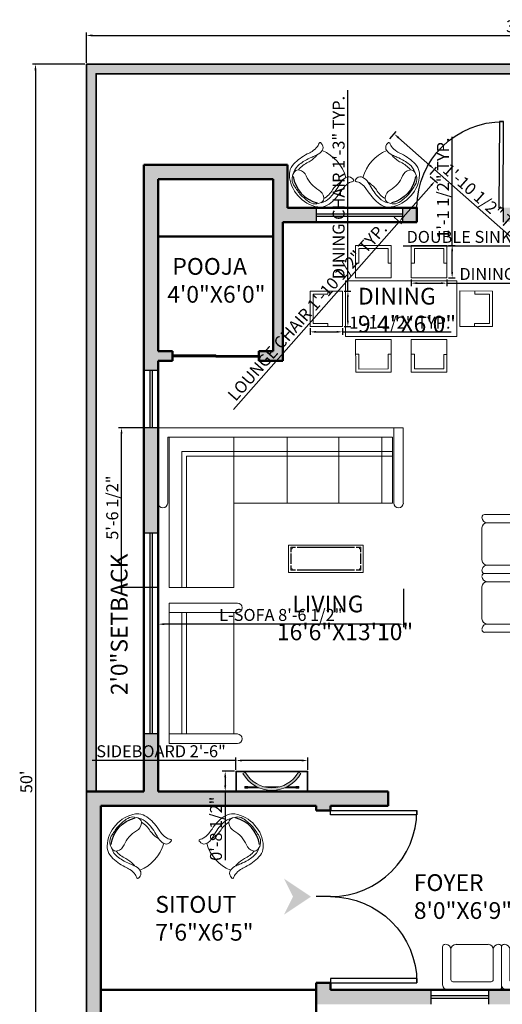
# Model space of a CAD drawing. Units: inches. Extents: x 2638 to 4577, y 1946 to 2619.
# Tile 2 of 8: x 2638 to 2839, y 2207 to 2619. Entities that reach past the tile are written whole.
import ezdxf

# ---------------------------------------------------------------- set-up
doc = ezdxf.new("R2010")
doc.units = ezdxf.units.IN
for name, color, linetype, lineweight in [('A-ANNO-DIMS', 2, 'Continuous', 18), ('A-ANNO-SYMB', 1, 'Continuous', 25), ('A-ANNO-TEXT', 7, 'Continuous', 25), ('A-AREA-IDEN', 7, 'Continuous', 25), ('A-DOOR', 4, 'Continuous', 25), ('A-FURN', 8, 'Continuous', 18), ('A-GLAZ', 4, 'Continuous', 25), ('A-WALL', 7, 'Continuous', 50), ('A-WALL-PATT', 8, 'Continuous', 13), ('aparador', 36, 'Continuous', 9), ('C-PROP', 1, 'Continuous', 35), ('C-PROP-PATT', 252, 'Continuous', 13), ('moveis', 254, 'Continuous', 5)]:
    doc.layers.add(name, color=color, linetype=linetype, lineweight=lineweight)
doc.layers.add('IFF-FURN-DETAIL', color=250, linetype='Continuous')
doc.styles.get("Standard").update_dxf_attribs({"font": 'arial.ttf'})
doc.dimstyles.new('ISO-25', dxfattribs={"dimtxt": 5, "dimasz": 2.5, "dimexe": 1.25, "dimexo": 0.625, "dimtad": 1, "dimdec": 1, "dimlunit": 3, "dimtxsty": 'Standard', "dimcen": 2.5, "dimclrt": 1, "dimadec": 0, "dimazin": 0, "dimtfac": 1, "dimtdec": 1, "dimtmove": 0, "dimatfit": 3, "dimfxl": 1, "dimarcsym": 0})

# ---------------------------------------------------------------- blocks, each defined once
blk = doc.blocks.new('*D1')
at = {"layer": 'A-ANNO-DIMS', "color": 0, "lineweight": -2, "transparency": 16777216}
for p, q in [((2665.41, 2600.78), (2665.41, 2613.44)), ((2667.91, 2612.19), (3022.91, 2612.19)), ((3025.41, 2600.78), (3025.41, 2613.44))]:
    blk.add_line(p, q, dxfattribs=at)
at = {"layer": 'A-ANNO-DIMS', "color": 0, "transparency": 16777216}
for points in [[(2667.91, 2612.61), (2667.91, 2611.77), (2665.41, 2612.19)], [(3022.91, 2612.61), (3022.91, 2611.77), (3025.41, 2612.19)]]:
    blk.add_solid(points, dxfattribs=at)
at = {"layer": 'Defpoints', "color": 0, "transparency": 16777216}
for p in [(3025.41, 2612.19), (2665.41, 2600.16), (3025.41, 2600.16)]:
    blk.add_point(p, dxfattribs=at)
at = {"layer": 'A-ANNO-DIMS', "color": 0, "transparency": 16777216, "insert": (2845.41, 2615.37), "char_height": 5, "attachment_point": 5}
blk.add_mtext("30'", dxfattribs=at)
blk = doc.blocks.new('*D2')
at = {"layer": 'A-ANNO-DIMS', "color": 0, "lineweight": -2, "transparency": 16777216}
for p, q in [((2664.78, 2600.16), (2642.86, 2600.16)), ((2644.11, 2597.66), (2644.11, 2002.66)), ((2664.78, 2000.16), (2642.86, 2000.16))]:
    blk.add_line(p, q, dxfattribs=at)
at = {"layer": 'A-ANNO-DIMS', "color": 0, "transparency": 16777216}
for points in [[(2643.7, 2597.66), (2644.53, 2597.66), (2644.11, 2600.16)], [(2643.7, 2002.66), (2644.53, 2002.66), (2644.11, 2000.16)]]:
    blk.add_solid(points, dxfattribs=at)
at = {"layer": 'Defpoints', "color": 0, "transparency": 16777216}
for p in [(2665.41, 2600.16), (2644.11, 2000.16), (2665.41, 2000.16)]:
    blk.add_point(p, dxfattribs=at)
at = {"layer": 'A-ANNO-DIMS', "color": 0, "transparency": 16777216, "insert": (2640.93, 2300.16), "char_height": 5, "attachment_point": 5, "rotation": 90}
blk.add_mtext("50'", dxfattribs=at)
blk = doc.blocks.new('*U4')
for p, q in [((0, 0), (0, -6)), ((36, 0), (36, -6))]:
    blk.add_line(p, q)
blk.add_lwpolyline([(0, 0), (0, 36), (1.75, 36), (1.75, 0)], close=True)
blk.add_arc((0, 0), 36, 0, 90)
blk = doc.blocks.new('Aparador ORGANICA Formatto')
at = {"layer": 'aparador', "ltscale": 0.3}
h = blk.add_hatch(color=256, dxfattribs=at)
h.dxf.hatch_style = 1
h.set_gradient(color1=(118, 213, 123), color2=(52, 168, 57), one_color=1, tint=0.43, name='INVCURVED')
h.paths.add_polyline_path([(0.8, 0.45), (-0.8, 0.45), (-0.8, 0), (0.8, 0)])
h.paths.add_polyline_path([(0.785, 0.435), (0.785, 0.015), (-0.785, 0.015), (-0.785, 0.435)], flags=16)
h.paths.add_polyline_path([(0.291, 0.37), (0.537, 0.37), (0.537, 0.376), (0.601, 0.376), (0.601, 0.37), (0.601, 0.35), (0.601, 0.344), (0.537, 0.344), (0.537, 0.35), (0.334, 0.35, -0.150336), (0.645, 0.049), (0.592, 0.02, 0.208852), (0.163, 0.35), (-0.163, 0.35, 0.208852), (-0.592, 0.02), (-0.645, 0.049, -0.150336), (-0.334, 0.35), (-0.537, 0.35), (-0.537, 0.344), (-0.601, 0.344), (-0.601, 0.35), (-0.601, 0.37), (-0.601, 0.376), (-0.537, 0.376), (-0.537, 0.37), (-0.291, 0.37, -0.206106)], flags=0)
h = blk.add_hatch(color=256, dxfattribs=at)
h.dxf.hatch_style = 1
h.set_gradient(color1=(135, 92, 69), color2=(0, 0, 0), one_color=1, name='INVCURVED')
h.paths.add_polyline_path([(-0.645, 0.049), (-0.592, 0.02, -0.590888), (0.592, 0.02), (0.645, 0.049, 0.590888)])
h = blk.add_hatch(color=256, dxfattribs=at)
h.dxf.hatch_style = 1
h.set_gradient(color1=(178, 189, 189), one_color=1, tint=1, name='CYLINDER')
h.paths.add_polyline_path([(-0.537, 0.376), (-0.601, 0.376), (-0.601, 0.37), (-0.537, 0.37)])
h.paths.add_polyline_path([(-0.537, 0.35), (-0.601, 0.35), (-0.601, 0.344), (-0.537, 0.344)])
h = blk.add_hatch(color=256, dxfattribs=at)
h.dxf.hatch_style = 1
h.set_gradient(color1=(118, 213, 123), color2=(31, 101, 35), one_color=1, tint=0.26, name='INVCURVED')
h.paths.add_polyline_path([(-0.291, 0.37), (-0.601, 0.37), (-0.601, 0.35), (-0.334, 0.35, -0.015999)])
h = blk.add_hatch(color=256, dxfattribs=at)
h.dxf.hatch_style = 1
h.set_gradient(color1=(118, 213, 123), color2=(31, 101, 35), one_color=1, tint=0.26, name='INVCURVED')
h.paths.add_polyline_path([(-0.163, 0.35), (0.163, 0.35, 0.122516)])
h = blk.add_hatch(color=256, dxfattribs=at)
h.dxf.hatch_style = 1
h.set_gradient(color1=(118, 213, 123), color2=(31, 101, 35), one_color=1, tint=0.26, name='INVCURVED')
h.paths.add_polyline_path([(0.601, 0.37), (0.291, 0.37, -0.015999), (0.334, 0.35), (0.601, 0.35)])
h = blk.add_hatch(color=256, dxfattribs=at)
h.dxf.hatch_style = 1
h.set_gradient(color1=(178, 189, 189), one_color=1, tint=1, name='CYLINDER')
h.paths.add_polyline_path([(0.601, 0.376), (0.537, 0.376), (0.537, 0.37), (0.601, 0.37)])
h.paths.add_polyline_path([(0.601, 0.35), (0.537, 0.35), (0.537, 0.344), (0.601, 0.344)])
for p, q in [((-0.592, 0.02), (-0.645, 0.049)), ((0.592, 0.02), (0.645, 0.049))]:
    blk.add_line(p, q, dxfattribs=at)
for points in [[(-0.601, 0.37), (-0.601, 0.376), (-0.537, 0.376), (-0.537, 0.37)], [(-0.537, 0.35), (-0.537, 0.344), (-0.601, 0.344), (-0.601, 0.35)], [(0.601, 0.37), (0.601, 0.376), (0.537, 0.376), (0.537, 0.37)], [(0.537, 0.35), (0.537, 0.344), (0.601, 0.344), (0.601, 0.35)]]:
    blk.add_lwpolyline(points, dxfattribs=at)
for radius in [0.736, 0.676]:
    blk.add_arc((0, -0.306), radius, 28.8434, 151.1566, dxfattribs=at)
at = {"layer": 'moveis', "ltscale": 0.3}
for p, q in [((-0.601, 0.37), (-0.601, 0.35)), ((-0.291, 0.37), (-0.601, 0.37)), ((-0.601, 0.35), (-0.334, 0.35)), ((-0.163, 0.35), (0.163, 0.35)), ((0.291, 0.37), (0.601, 0.37)), ((0.601, 0.35), (0.334, 0.35)), ((0.601, 0.37), (0.601, 0.35))]:
    blk.add_line(p, q, dxfattribs=at)
for points in [[(-0.8, 0), (0.8, 0), (0.8, 0.45), (-0.8, 0.45)], [(-0.785, 0.015), (0.785, 0.015), (0.785, 0.435), (-0.785, 0.435)]]:
    blk.add_lwpolyline(points, close=True, dxfattribs=at)
blk = doc.blocks.new('TABLE-30A')
at = {"color": 0, "linetype": 'ByBlock'}
for p, q in [((0, 0), (0, 0.55)), ((0, 0.55), (1.5, 0.55)), ((0.051, 0.508), (0.042, 0.499)), ((0.042, 0.499), (0.042, 0.478)), ((0.042, 0.478), (0.072, 0.478)), ((0.042, 0.478), (0.042, 0.41)), ((0.072, 0.508), (0.051, 0.508)), ((0.051, 0.478), (0.051, 0.41)), ((0.072, 0.478), (0.072, 0.508)), ((0.072, 0.508), (0.14, 0.508)), ((0.072, 0.499), (0.14, 0.499)), ((1.331, 0.508), (0.169, 0.508)), ((1.331, 0.499), (0.169, 0.499)), ((1.428, 0.508), (1.36, 0.508)), ((1.428, 0.499), (1.36, 0.499)), ((1.428, 0.508), (1.428, 0.478)), ((1.449, 0.508), (1.428, 0.508)), ((1.428, 0.478), (1.458, 0.478)), ((1.458, 0.499), (1.449, 0.508)), ((1.449, 0.478), (1.449, 0.41)), ((1.458, 0.478), (1.458, 0.499)), ((1.458, 0.478), (1.458, 0.41)), ((1.5, 0.55), (1.5, 0)), ((0.042, 0.169), (0.042, 0.381)), ((0.051, 0.169), (0.051, 0.381)), ((1.449, 0.381), (1.449, 0.169)), ((1.458, 0.381), (1.458, 0.169)), ((1.5, 0), (0, 0)), ((0.042, 0.072), (0.042, 0.14)), ((0.042, 0.072), (0.042, 0.051)), ((0.072, 0.072), (0.042, 0.072)), ((0.042, 0.051), (0.051, 0.042)), ((0.051, 0.072), (0.051, 0.14)), ((0.051, 0.042), (0.072, 0.042)), ((0.072, 0.042), (0.072, 0.072)), ((0.072, 0.051), (0.14, 0.051)), ((0.072, 0.042), (0.14, 0.042)), ((0.169, 0.051), (1.331, 0.051)), ((0.169, 0.042), (1.331, 0.042)), ((1.428, 0.051), (1.36, 0.051)), ((1.428, 0.042), (1.36, 0.042)), ((1.428, 0.072), (1.428, 0.042)), ((1.458, 0.072), (1.428, 0.072)), ((1.428, 0.042), (1.449, 0.042)), ((1.449, 0.072), (1.449, 0.14)), ((1.449, 0.042), (1.458, 0.051)), ((1.458, 0.072), (1.458, 0.14)), ((1.458, 0.051), (1.458, 0.072))]:
    blk.add_line(p, q, dxfattribs=at)
blk = doc.blocks.new('12')
at = {"color": 0}
for p, q in [((5656.26, 3021.25), (5553.9, 3021.25)), ((5553.9, 3021.25), (5553.9, 2989.76)), ((5557.83, 3021.25), (5557.83, 2989.76)), ((5652.32, 3017.31), (5558.49, 3017.31)), ((5558.49, 3017.31), (5558.49, 2989.76)), ((5562.89, 3017.31), (5562.89, 2989.76)), ((5580.8, 3017.31), (5580.8, 2989.76)), ((5602.45, 3017.31), (5602.45, 2989.76)), ((5624.76, 3017.31), (5624.76, 2954.53)), ((5651.66, 3017.31), (5651.66, 2954.53)), ((5652.32, 2989.76), (5652.32, 3017.31)), ((5656.26, 2989.76), (5656.26, 3021.25)), ((5646.42, 3011.41), (5558.49, 3011.41)), ((5644.45, 3009.44), (5558.49, 3009.44)), ((5644.45, 2954.53), (5644.45, 3009.44)), ((5646.42, 2954.53), (5646.42, 3011.41)), ((5624.76, 2995), (5624.76, 2954.53)), ((5558.49, 2989.76), (5624.76, 2989.76)), ((5651.66, 2954.53), (5624.76, 2954.53))]:
    blk.add_line(p, q, dxfattribs=at)
for centre in [(5555.86, 2989.76), (5654.29, 2989.76)]:
    blk.add_arc(centre, 1.97, 180, 0, dxfattribs=at)
at = {"xscale": -20.70834898381633, "yscale": 20.70834898381633, "zscale": 20.70834898381633}
blk.add_blockref('TABLE-30A', (5601.8, 2960.82), dxfattribs=at)
blk = doc.blocks.new('ILNG95')
for points in [[(120, 308, -0.32971), (51, 384, -0.036099), (50, 422, -0.497733), (75, 439, -0.070621), (96, 429, 0.101868), (133, 414, 0.091794), (259, 412, 0.024114), (351, 433, -0.090294), (638, 458, -0.132412), (775, 407, -0.068618), (816, 368, -0.184346), (943, 0, 1.803905)], [(120, 308, 0.138132), (244, 313, 0.001085), (325, 339, -0.034227), (462, 375, -0.033255), (567, 387, -0.137428), (727, 350, -4.561553)], [(120, 308, 0.138132), (244, 313, 0.001085), (325, 339, -0.034227), (462, 375, -0.033255), (567, 387, -0.137428), (727, 350, -4.561553)], [(639, 0, 0.078302), (612, 161, -0.233633), (633, 315, -0.28763), (710, 349, -0.317923), (875, 193, -0.032882), (900, 0, 1.140397)], [(639, 0, 0.078302), (612, 161, -0.233633), (633, 315, -0.28763), (710, 349, -0.317923), (875, 193, -0.032882), (900, 0, 1.140397)], [(235, 308, 0.064243), (394, 307, 0.04414), (433, 315, -0.118032), (643, 329, -6.296816)], [(235, 308, 0.064243), (394, 307, 0.04414), (433, 315, -0.118032), (643, 329, -6.296816)], [(120, -308, 0.32971), (51, -384, 0.036099), (50, -422, 0.497733), (75, -439, 0.070621), (96, -429, -0.101868), (133, -414, -0.091794), (259, -412, -0.024114), (351, -433, 0.090294), (638, -458, 0.132412), (775, -407, 0.068618), (816, -368, 0.184346), (943, 0, -1.803905)], [(639, 0, -0.078302), (612, -161, 0.233633), (633, -315, 0.28763), (710, -349, 0.317923), (875, -193, 0.032882), (900, 0, -1.140397)], [(639, 0, -0.078302), (612, -161, 0.233633), (633, -315, 0.28763), (710, -349, 0.317923), (875, -193, 0.032882), (900, 0, -1.140397)], [(120, -308, -0.138132), (244, -313, -0.001085), (325, -339, 0.034227), (462, -375, 0.033255), (567, -387, 0.137428), (727, -350, 4.561553)], [(120, -308, -0.138132), (244, -313, -0.001085), (325, -339, 0.034227), (462, -375, 0.033255), (567, -387, 0.137428), (727, -350, 4.561553)], [(235, -308, -0.064243), (394, -307, -0.04414), (433, -315, 0.118032), (643, -329, 6.296816)], [(235, -308, -0.064243), (394, -307, -0.04414), (433, -315, 0.118032), (643, -329, 6.296816)]]:
    blk.add_lwpolyline(points, format="xyb")
blk.add_arc((759, 1), 709, 154.3281, 205.801)
at = {"layer": 'IFF-FURN-DETAIL'}
blk.add_arc((326, -2), 549, 326.8997, 34.6691, dxfattribs=at)
blk.add_arc((326, -2), 549, 326.8997, 34.6691, dxfattribs=at)
blk = doc.blocks.new('sofa-27')
at = {"color": 0, "linetype": 'ByBlock'}
for p, q in [((-0.059, 0.059), (-0.059, 0.49)), ((0.035, 0.118), (0.035, 0.461)), ((0.094, 0.52), (0.459, 0.52)), ((0.518, 0.118), (0.518, 0.461)), ((0.613, 0.03), (0.613, 0.49)), ((0.583, 0), (0, 0)), ((0.494, 0.094), (0.059, 0.094))]:
    blk.add_line(p, q, dxfattribs=at)
for centre, radius, start, end in [((-0.03, 0.49), 0.0295, 90, 180), ((-0.024, 0.461), 0.0591, 360, 90), ((0.094, 0.461), 0.0591, 90, 180), ((0.459, 0.461), 0.0591, 0, 90), ((0.577, 0.461), 0.0591, 90, 180), ((0.583, 0.49), 0.0295, 0, 90), ((0.059, 0.118), 0.0236, 180, 270), ((0.494, 0.118), 0.0236, 270, 0), ((0, 0.059), 0.0591, 180, 270), ((0.583, 0.03), 0.0295, 270, 0)]:
    blk.add_arc(centre, radius, start, end, dxfattribs=at)
blk = doc.blocks.new('CHAIR-DINING')
for p, q in [((2758.8, 2505.34), (2772.37, 2505.34)), ((2758.8, 2490.5), (2758.8, 2505.34)), ((2760.08, 2504.06), (2766.22, 2504.06)), ((2760.08, 2491.82), (2760.08, 2504.06)), ((2766.22, 2504.06), (2766.22, 2505.34)), ((2772.37, 2490.5), (2772.37, 2505.34)), ((2758.8, 2490.5), (2772.37, 2490.5)), ((2766.22, 2491.82), (2760.08, 2491.82)), ((2766.22, 2490.5), (2766.22, 2491.82))]:
    blk.add_line(p, q)
blk = doc.blocks.new('CHAIR-DINING-B')
for p, q in [((2801.09, 2524.41), (2815.93, 2524.41)), ((2801.09, 2524.41), (2801.09, 2510.85)), ((2815.93, 2524.41), (2815.93, 2510.85)), ((2802.37, 2523.09), (2814.65, 2523.09)), ((2802.37, 2516.99), (2802.37, 2523.09)), ((2814.65, 2523.09), (2814.65, 2516.99)), ((2801.09, 2516.99), (2802.37, 2516.99)), ((2814.65, 2516.99), (2815.93, 2516.99)), ((2801.09, 2510.85), (2815.93, 2510.85))]:
    blk.add_line(p, q)
blk = doc.blocks.new('WIN-36')
for p, q in [((2761.41, 2540.16), (2761.41, 2534.16)), ((2797.41, 2540.16), (2797.41, 2534.16)), ((2761.41, 2537.66), (2797.41, 2537.66)), ((2761.41, 2536.66), (2797.41, 2536.66))]:
    blk.add_line(p, q)
blk = doc.blocks.new('WIN-24')
for p, q in [((2905.41, 2558.16), (2905.41, 2552.16)), ((2929.41, 2558.16), (2929.41, 2552.16)), ((2905.41, 2555.66), (2929.41, 2555.66)), ((2905.41, 2554.66), (2929.41, 2554.66))]:
    blk.add_line(p, q)
blk = doc.blocks.new('WIN-84')
for p, q in [((2695.41, 2404.16), (2689.41, 2404.16)), ((2691.91, 2404.16), (2691.91, 2320.16)), ((2692.91, 2404.16), (2692.91, 2320.16)), ((2695.41, 2320.16), (2689.41, 2320.16))]:
    blk.add_line(p, q)
blk = doc.blocks.new('*D57')
at = {"layer": 'A-ANNO-DIMS', "color": 0, "lineweight": -2, "transparency": 16777216}
for p, q in [((2808.96, 2553.23), (2811.99, 2550.56)), ((2809.4, 2549.51), (2797.66, 2536.2)), ((2793.92, 2536.17), (2796.95, 2533.5)), ((2796.01, 2534.32), (2726.78, 2455.83))]:
    blk.add_line(p, q, dxfattribs=at)
at = {"layer": 'A-ANNO-DIMS', "color": 0, "transparency": 16777216}
for points in [[(2809.09, 2549.78), (2809.71, 2549.23), (2811.05, 2551.38)], [(2797.35, 2536.47), (2797.97, 2535.92), (2796.01, 2534.32)]]:
    blk.add_solid(points, dxfattribs=at)
at = {"layer": 'Defpoints', "color": 0, "transparency": 16777216}
for p in [(2808.5, 2553.64), (2793.45, 2536.58), (2796.01, 2534.32)]:
    blk.add_point(p, dxfattribs=at)
at = {"layer": 'A-ANNO-DIMS', "color": 1, "transparency": 16777216, "insert": (2758.16, 2496.27), "char_height": 5, "attachment_point": 5, "rotation": 48.5881}
blk.add_mtext('LOUNGE CHAIR 1\'-10 1/2" TYP.', dxfattribs=at)
blk = doc.blocks.new('*D58')
at = {"layer": 'A-ANNO-DIMS', "color": 0, "lineweight": -2, "transparency": 16777216}
for p, q in [((2792.08, 2568.95), (2794.75, 2571.98)), ((2795.8, 2569.39), (2808.88, 2557.85)), ((2808.91, 2554.11), (2811.58, 2557.14)), ((2810.75, 2556.2), (2847.72, 2523.59))]:
    blk.add_line(p, q, dxfattribs=at)
at = {"layer": 'A-ANNO-DIMS', "color": 0, "transparency": 16777216}
for points in [[(2796.07, 2569.7), (2795.52, 2569.08), (2793.92, 2571.04)], [(2809.15, 2558.16), (2808.6, 2557.54), (2810.75, 2556.2)]]:
    blk.add_solid(points, dxfattribs=at)
at = {"layer": 'Defpoints', "color": 0, "transparency": 16777216}
for p in [(2791.66, 2568.48), (2810.75, 2556.2), (2808.5, 2553.64)]:
    blk.add_point(p, dxfattribs=at)
at = {"layer": 'A-ANNO-DIMS', "color": 1, "transparency": 16777216, "insert": (2832.3, 2541.48), "char_height": 5, "attachment_point": 5, "rotation": 318.5881}
blk.add_mtext('1\'-10 1/2" TYP.', dxfattribs=at)
blk = doc.blocks.new('*D63')
at = {"layer": 'A-ANNO-DIMS', "color": 0, "lineweight": -2, "transparency": 16777216}
for p, q in [((2774.6, 2505.34), (2774.6, 2589.38)), ((2772.99, 2505.34), (2775.85, 2505.34)), ((2774.6, 2493), (2774.6, 2502.84)), ((2772.99, 2490.5), (2775.85, 2490.5))]:
    blk.add_line(p, q, dxfattribs=at)
at = {"layer": 'A-ANNO-DIMS', "color": 0, "transparency": 16777216}
for points in [[(2774.18, 2502.84), (2775.01, 2502.84), (2774.6, 2505.34)], [(2774.18, 2493), (2775.01, 2493), (2774.6, 2490.5)]]:
    blk.add_solid(points, dxfattribs=at)
at = {"layer": 'Defpoints', "color": 0, "transparency": 16777216}
for p in [(2772.37, 2505.34), (2774.6, 2505.34), (2772.37, 2490.5)]:
    blk.add_point(p, dxfattribs=at)
at = {"layer": 'A-ANNO-DIMS', "color": 1, "transparency": 16777216, "insert": (2771.38, 2548.61), "char_height": 5, "attachment_point": 5, "rotation": 90}
blk.add_mtext('DINING CHAIR 1\'-3" TYP.', dxfattribs=at)
blk = doc.blocks.new('*D64')
at = {"layer": 'A-ANNO-DIMS', "color": 0, "lineweight": -2, "transparency": 16777216}
for p, q in [((2758.8, 2489.88), (2758.8, 2487.03)), ((2761.3, 2488.28), (2769.87, 2488.28)), ((2772.37, 2489.88), (2772.37, 2487.03)), ((2772.37, 2488.28), (2817.78, 2488.28))]:
    blk.add_line(p, q, dxfattribs=at)
at = {"layer": 'A-ANNO-DIMS', "color": 0, "transparency": 16777216}
for points in [[(2761.3, 2488.69), (2761.3, 2487.86), (2758.8, 2488.28)], [(2769.87, 2488.69), (2769.87, 2487.86), (2772.37, 2488.28)]]:
    blk.add_solid(points, dxfattribs=at)
at = {"layer": 'Defpoints', "color": 0, "transparency": 16777216}
for p in [(2758.8, 2490.5), (2772.37, 2490.5), (2772.37, 2488.28)]:
    blk.add_point(p, dxfattribs=at)
at = {"layer": 'A-ANNO-DIMS', "color": 1, "transparency": 16777216, "insert": (2796.32, 2491.49), "char_height": 5, "attachment_point": 5}
blk.add_mtext('1\'-1 1/2" TYP.', dxfattribs=at)
blk = doc.blocks.new('*D65')
at = {"layer": 'A-ANNO-DIMS', "color": 0, "lineweight": -2, "transparency": 16777216}
for p, q in [((2801.09, 2510.22), (2801.09, 2507.37)), ((2803.59, 2508.62), (2813.43, 2508.62)), ((2815.93, 2510.22), (2815.93, 2507.37)), ((2815.93, 2508.62), (2906.57, 2508.62))]:
    blk.add_line(p, q, dxfattribs=at)
at = {"layer": 'A-ANNO-DIMS', "color": 0, "transparency": 16777216}
for points in [[(2803.59, 2509.04), (2803.59, 2508.21), (2801.09, 2508.62)], [(2813.43, 2509.04), (2813.43, 2508.21), (2815.93, 2508.62)]]:
    blk.add_solid(points, dxfattribs=at)
at = {"layer": 'Defpoints', "color": 0, "transparency": 16777216}
for p in [(2801.09, 2510.85), (2815.93, 2510.85), (2815.93, 2508.62)]:
    blk.add_point(p, dxfattribs=at)
at = {"layer": 'A-ANNO-DIMS', "color": 1, "transparency": 16777216, "insert": (2862.5, 2511.84), "char_height": 5, "attachment_point": 5}
blk.add_mtext('DINING CHAIR B 1\'-3" TYP.', dxfattribs=at)
blk = doc.blocks.new('*D66')
at = {"layer": 'A-ANNO-DIMS', "color": 0, "lineweight": -2, "transparency": 16777216}
for p, q in [((2818.16, 2524.41), (2818.16, 2569.82)), ((2816.56, 2524.41), (2819.41, 2524.41)), ((2818.16, 2513.35), (2818.16, 2521.91)), ((2816.56, 2510.85), (2819.41, 2510.85))]:
    blk.add_line(p, q, dxfattribs=at)
at = {"layer": 'A-ANNO-DIMS', "color": 0, "transparency": 16777216}
for points in [[(2817.74, 2521.91), (2818.57, 2521.91), (2818.16, 2524.41)], [(2817.74, 2513.35), (2818.57, 2513.35), (2818.16, 2510.85)]]:
    blk.add_solid(points, dxfattribs=at)
at = {"layer": 'Defpoints', "color": 0, "transparency": 16777216}
for p in [(2815.93, 2524.41), (2818.16, 2524.41), (2815.93, 2510.85)]:
    blk.add_point(p, dxfattribs=at)
at = {"layer": 'A-ANNO-DIMS', "color": 1, "transparency": 16777216, "insert": (2814.95, 2548.36), "char_height": 5, "attachment_point": 5, "rotation": 90}
blk.add_mtext('1\'-1 1/2" TYP.', dxfattribs=at)
blk = doc.blocks.new('*D77')
at = {"layer": 'A-ANNO-DIMS', "color": 0, "lineweight": -2, "transparency": 16777216}
for p, q in [((2727.86, 2305.21), (2727.86, 2310.33)), ((2757.84, 2305.21), (2757.84, 2310.33)), ((2727.86, 2309.08), (2667.76, 2309.08)), ((2755.34, 2309.08), (2730.36, 2309.08))]:
    blk.add_line(p, q, dxfattribs=at)
at = {"layer": 'A-ANNO-DIMS', "color": 0, "transparency": 16777216}
for points in [[(2730.36, 2309.5), (2730.36, 2308.67), (2727.86, 2309.08)], [(2755.34, 2309.5), (2755.34, 2308.67), (2757.84, 2309.08)]]:
    blk.add_solid(points, dxfattribs=at)
at = {"layer": 'Defpoints', "color": 0, "transparency": 16777216}
for p in [(2727.86, 2309.08), (2727.86, 2304.59), (2757.84, 2304.59)]:
    blk.add_point(p, dxfattribs=at)
at = {"layer": 'A-ANNO-DIMS', "color": 1, "transparency": 16777216, "insert": (2696.56, 2312.3), "char_height": 5, "attachment_point": 5}
blk.add_mtext('SIDEBOARD 2\'-6"', dxfattribs=at)
blk = doc.blocks.new('*D78')
at = {"layer": 'A-ANNO-DIMS', "color": 0, "lineweight": -2, "transparency": 16777216}
for p, q in [((2727.24, 2304.59), (2722.12, 2304.59)), ((2723.37, 2302.09), (2723.37, 2298.66)), ((2727.24, 2296.16), (2722.12, 2296.16)), ((2723.37, 2296.16), (2723.37, 2267.46))]:
    blk.add_line(p, q, dxfattribs=at)
at = {"layer": 'A-ANNO-DIMS', "color": 0, "transparency": 16777216}
for points in [[(2722.95, 2302.09), (2723.78, 2302.09), (2723.37, 2304.59)], [(2722.95, 2298.66), (2723.78, 2298.66), (2723.37, 2296.16)]]:
    blk.add_solid(points, dxfattribs=at)
at = {"layer": 'Defpoints', "color": 0, "transparency": 16777216}
for p in [(2727.86, 2304.59), (2723.37, 2296.16), (2727.86, 2296.16)]:
    blk.add_point(p, dxfattribs=at)
at = {"layer": 'A-ANNO-DIMS', "color": 1, "transparency": 16777216, "insert": (2720.16, 2280.56), "char_height": 5, "attachment_point": 5, "rotation": 90}
blk.add_mtext('0\'-8 1/2"', dxfattribs=at)
blk = doc.blocks.new('*D83')
at = {"layer": 'A-ANNO-DIMS', "color": 0, "lineweight": -2, "transparency": 16777216}
for p, q in [((2695.4, 2380.81), (2695.4, 2364.83)), ((2797.77, 2380.81), (2797.77, 2364.83)), ((2795.27, 2366.08), (2697.9, 2366.08))]:
    blk.add_line(p, q, dxfattribs=at)
at = {"layer": 'A-ANNO-DIMS', "color": 0, "transparency": 16777216}
for points in [[(2697.9, 2366.49), (2697.9, 2365.66), (2695.4, 2366.08)], [(2795.27, 2366.49), (2795.27, 2365.66), (2797.77, 2366.08)]]:
    blk.add_solid(points, dxfattribs=at)
at = {"layer": 'Defpoints', "color": 0, "transparency": 16777216}
for p in [(2695.4, 2381.43), (2797.77, 2381.43), (2695.4, 2366.08)]:
    blk.add_point(p, dxfattribs=at)
at = {"layer": 'A-ANNO-DIMS', "color": 1, "transparency": 16777216, "insert": (2746.58, 2369.29), "char_height": 5, "attachment_point": 5}
blk.add_mtext('L-SOFA 8\'-6 1/2"', dxfattribs=at)
blk = doc.blocks.new('*D84')
at = {"layer": 'A-ANNO-DIMS', "color": 0, "lineweight": -2, "transparency": 16777216}
for p, q in [((2694.78, 2448.16), (2678.8, 2448.16)), ((2680.05, 2383.93), (2680.05, 2445.66)), ((2694.78, 2381.43), (2678.8, 2381.43))]:
    blk.add_line(p, q, dxfattribs=at)
at = {"layer": 'A-ANNO-DIMS', "color": 0, "transparency": 16777216}
for points in [[(2679.63, 2445.66), (2680.46, 2445.66), (2680.05, 2448.16)], [(2679.63, 2383.93), (2680.46, 2383.93), (2680.05, 2381.43)]]:
    blk.add_solid(points, dxfattribs=at)
at = {"layer": 'Defpoints', "color": 0, "transparency": 16777216}
for p in [(2680.05, 2448.16), (2695.4, 2448.16), (2695.4, 2381.43)]:
    blk.add_point(p, dxfattribs=at)
at = {"layer": 'A-ANNO-DIMS', "color": 1, "transparency": 16777216, "insert": (2676.84, 2414.79), "char_height": 5, "attachment_point": 5, "rotation": 90}
blk.add_mtext('5\'-6 1/2"', dxfattribs=at)
blk = doc.blocks.new('*D85')
at = {"layer": 'A-ANNO-DIMS', "color": 0, "lineweight": -2, "transparency": 16777216}
for p, q in [((2863.41, 2528.9), (2863.41, 2522.87)), ((2899.41, 2528.9), (2899.41, 2522.87)), ((2863.41, 2524.12), (2797.71, 2524.12)), ((2896.91, 2524.12), (2865.91, 2524.12))]:
    blk.add_line(p, q, dxfattribs=at)
at = {"layer": 'A-ANNO-DIMS', "color": 0, "transparency": 16777216}
for points in [[(2865.91, 2524.54), (2865.91, 2523.7), (2863.41, 2524.12)], [(2896.91, 2524.54), (2896.91, 2523.7), (2899.41, 2524.12)]]:
    blk.add_solid(points, dxfattribs=at)
at = {"layer": 'Defpoints', "color": 0, "transparency": 16777216}
for p in [(2863.41, 2529.52), (2899.41, 2529.52), (2863.41, 2524.12)]:
    blk.add_point(p, dxfattribs=at)
at = {"layer": 'A-ANNO-DIMS', "color": 1, "transparency": 16777216, "insert": (2829.31, 2527.33), "char_height": 5, "attachment_point": 5}
blk.add_mtext('DOUBLE SINK 3\'-0"', dxfattribs=at)

msp = doc.modelspace()

# ---------------------------------------------------------------- hatches: boundary and pattern name
at = {"layer": 'A-ANNO-SYMB', "transparency": 33554687}
h = msp.add_hatch(color=256, dxfattribs=at)
h.dxf.hatch_style = 1
h.paths.add_polyline_path([(2751.65, 2252.16), (2747.88, 2244.61), (2759.2, 2252.16), (2747.88, 2259.71)])
at = {"layer": 'A-WALL-PATT', "transparency": 33554687}
h = msp.add_hatch(color=256, dxfattribs=at)
h.dxf.hatch_style = 1
h.paths.add_polyline_path([(2749.41, 2558.16), (2689.41, 2558.16), (2689.41, 2472.16), (2695.41, 2472.16), (2695.41, 2476.16), (2701.41, 2476.16), (2701.41, 2480.16), (2695.41, 2480.16), (2695.41, 2552.16), (2743.41, 2552.16), (2743.41, 2480.16), (2737.41, 2480.16), (2737.41, 2476.16), (2747.41, 2476.16), (2747.41, 2534.16), (2761.41, 2534.16), (2761.41, 2540.16), (2749.41, 2540.16)])
h.paths.add_polyline_path([(2803.41, 2540.16), (2797.41, 2540.16), (2797.41, 2534.16), (2803.41, 2534.16)])
h.paths.add_polyline_path([(2905.41, 2558.16), (2857.41, 2558.16), (2857.41, 2540.16), (2839.44, 2540.16), (2839.44, 2540.16), (2839.41, 2534.26), (2839.41, 2534.16), (2859.41, 2534.16), (2859.41, 2516.16), (2863.41, 2516.16), (2863.41, 2552.16), (2905.41, 2552.16)])
h.paths.add_polyline_path([(3001.41, 2558.16), (2929.41, 2558.16), (2929.41, 2552.16), (2995.41, 2552.16), (2995.41, 2522.16), (3001.41, 2522.16)])
h.paths.add_polyline_path([(3001.41, 2486.16), (2995.41, 2486.16), (2995.41, 2426.16), (2881.41, 2426.16), (2881.41, 2422.16), (2995.41, 2422.16), (2995.41, 2418.91), (3001.41, 2418.91)])
h.paths.add_polyline_path([(3001.41, 2382.91), (2995.41, 2382.91), (2995.41, 2336.41), (3001.41, 2336.41)])
h.paths.add_polyline_path([(3001.41, 2300.41), (2995.41, 2300.41), (2995.41, 2296.16), (2908.41, 2296.16), (2908.41, 2292.16), (2913.41, 2292.16), (2913.41, 2264.16), (2917.41, 2264.16), (2917.41, 2292.16), (2995.41, 2292.16), (2995.41, 2274.16), (3001.41, 2274.16)])
h.paths.add_polyline_path([(3001.41, 2250.16), (2995.41, 2250.16), (2995.41, 2232.16), (2917.41, 2232.16), (2917.41, 2234.16), (2913.41, 2234.16), (2913.41, 2228.16), (2995.41, 2228.16), (2995.41, 2096.16), (3001.41, 2096.16)])
h.paths.add_polyline_path([(3001.41, 2060.16), (2995.41, 2060.16), (2995.41, 2024.16), (2971.41, 2024.16), (2971.41, 2018.16), (3001.41, 2018.16)])
h.paths.add_polyline_path([(2869.41, 2292.16), (2872.41, 2292.16), (2872.41, 2296.16), (2863.41, 2296.16), (2863.41, 2213.16), (2833.41, 2213.16), (2833.41, 2207.16), (2863.41, 2207.16), (2863.41, 2018.16), (2893.41, 2018.16), (2893.41, 2024.16), (2869.41, 2024.16)])
h.paths.add_polyline_path([(2809.41, 2213.16), (2767.41, 2213.16), (2767.41, 2216.16), (2761.41, 2216.16), (2761.41, 2207.16), (2809.41, 2207.16)])
h.paths.add_polyline_path([(2671.41, 2290.16), (2761.41, 2290.16), (2761.41, 2288.16), (2767.41, 2288.16), (2767.41, 2290.16), (2791.41, 2290.16), (2791.41, 2296.16), (2695.41, 2296.16), (2695.41, 2320.16), (2689.41, 2320.16), (2689.41, 2296.16), (2665.41, 2296.16), (2665.41, 2193.16), (2671.41, 2193.16)])
h.paths.add_polyline_path([(2695.41, 2448.16), (2689.41, 2448.16), (2689.41, 2404.16), (2695.41, 2404.16)])
at = {"layer": 'C-PROP-PATT', "transparency": 33554687}
h = msp.add_hatch(color=256, dxfattribs=at)
h.dxf.hatch_style = 1
h.paths.add_polyline_path([(3025.41, 2600.16), (2665.41, 2600.16), (2665.41, 2296.16), (2669.41, 2296.16), (2669.41, 2596.16), (3021.41, 2596.16), (3021.41, 2004.16), (2863.41, 2004.16), (2863.41, 2000.16), (3025.41, 2000.16)])
h.paths.add_polyline_path([(2669.41, 2193.16), (2665.41, 2193.16), (2665.41, 2000.16), (2669.41, 2000.16)], flags=17)

# ---------------------------------------------------------------- linework, layer by layer
at = {"layer": 'A-FURN'}
for p, q in [((2773.65, 2509.57), (2820.12, 2509.57)), ((2773.65, 2486.31), (2773.65, 2509.57)), ((2820.12, 2509.57), (2820.12, 2486.31)), ((2820.12, 2486.31), (2773.65, 2486.31)), ((2701.41, 2478.66), (2719.41, 2478.66)), ((2719.41, 2478.66), (2719.41, 2477.66)), ((2719.41, 2477.66), (2737.41, 2477.66)), ((2700, 2316.24), (2700, 2374.9)), ((2700, 2374.9), (2728.49, 2374.9)), ((2700, 2370.96), (2726.9, 2370.96)), ((2700, 2370.96), (2728.49, 2370.96)), ((2705.24, 2370.96), (2705.24, 2320.17)), ((2707.21, 2370.96), (2707.21, 2320.17)), ((2726.9, 2320.17), (2726.9, 2370.96)), ((2700, 2320.17), (2726.9, 2320.17)), ((2700, 2320.17), (2728.49, 2320.17)), ((2700, 2316.24), (2728.49, 2316.24))]:
    msp.add_line(p, q, dxfattribs=at)
for centre in [(2728.49, 2372.93), (2728.49, 2318.2)]:
    msp.add_arc(centre, 1.97, 270, 90, dxfattribs=at)
at = {"layer": 'A-WALL'}
for p, q in [((2689.41, 2558.16), (2749.41, 2558.16)), ((2689.41, 2296.16), (2689.41, 2558.16)), ((2749.41, 2540.16), (2749.41, 2558.16)), ((2695.41, 2552.16), (2743.41, 2552.16)), ((2695.41, 2480.16), (2695.41, 2552.16)), ((2743.41, 2480.16), (2743.41, 2552.16)), ((2749.41, 2540.16), (2803.41, 2540.16)), ((2803.41, 2540.16), (2803.41, 2534.16)), ((2747.41, 2476.16), (2747.41, 2534.16)), ((2747.41, 2534.16), (2803.41, 2534.16)), ((2695.41, 2528.16), (2743.41, 2528.16)), ((2695.41, 2480.16), (2701.41, 2480.16)), ((2701.41, 2480.16), (2701.41, 2476.16)), ((2701.41, 2478.16), (2737.41, 2478.16)), ((2737.41, 2480.16), (2737.41, 2476.16)), ((2737.41, 2480.16), (2743.41, 2480.16)), ((2695.41, 2296.16), (2695.41, 2476.16)), ((2695.41, 2476.16), (2701.41, 2476.16)), ((2737.41, 2476.16), (2747.41, 2476.16)), ((2689.41, 2296.16), (2665.41, 2296.16)), ((2791.41, 2296.16), (2695.41, 2296.16)), ((2791.41, 2296.16), (2791.41, 2290.16)), ((2671.41, 2193.16), (2671.41, 2290.16)), ((2761.41, 2290.16), (2671.41, 2290.16)), ((2761.41, 2290.16), (2761.41, 2288.16)), ((2791.41, 2290.16), (2767.41, 2290.16)), ((2767.41, 2290.16), (2767.41, 2288.16)), ((2767.41, 2288.16), (2761.41, 2288.16)), ((2767.41, 2216.16), (2761.41, 2216.16)), ((2761.41, 2216.16), (2761.41, 2193.16)), ((2767.41, 2216.16), (2767.41, 2213.16)), ((2761.41, 2213.16), (2671.41, 2213.16)), ((2863.41, 2213.16), (2767.41, 2213.16))]:
    msp.add_line(p, q, dxfattribs=at)
at = {"layer": 'C-PROP'}
for points in [[(2669.41, 2000.16), (2665.41, 2000.16), (2665.41, 2600.16), (3025.41, 2600.16), (3025.41, 2000.16), (2863.41, 2000.16)], [(2669.41, 2296.16), (2669.41, 2596.16), (3021.41, 2596.16), (3021.41, 2004.16), (2863.41, 2004.16)]]:
    msp.add_lwpolyline(points, dxfattribs=at)

# ---------------------------------------------------------------- block references
at = {"layer": 'A-DOOR', "xscale": -1}
for p, rotation in [((2839.44, 2540.16), 359.6786649249896), ((2767.41, 2216.16), 270)]:
    msp.add_blockref('*U4', p, dxfattribs=dict(at, rotation=rotation))
at = {"layer": 'A-DOOR', "rotation": 270}
msp.add_blockref('*U4', (2767.41, 2288.16), dxfattribs=at)
at = {"layer": 'A-FURN'}
for name, p, xscale, yscale, zscale, rotation in [('ILNG95', (2771.02, 2560.38), 0.0243705291132055, 0.0243705291132055, 0.0243705291132055, 221.4118781376283), ('ILNG95', (2783.66, 2560.38), -0.0243705291132055, 0.0243705291132055, 0.0243705291132055, 138.5881218623715), ('sofa-27', (2849.68, 2389.46), 36.66436083614781, 36.66436083614781, 36.66436083614781, 90), ('sofa-27', (2849.68, 2364.84), 36.66436083614781, 36.66436083614781, 36.66436083614781, 90), ('Aparador ORGANICA Formatto', (2742.85, 2304.59), 18.73617255462838, 18.73617255462838, 18.73617255462838, 180), ('ILNG95', (2694.9, 2266.86), -0.0243705291132055, 0.0243705291132055, 0.0243705291132055, 318.5881218623716), ('ILNG95', (2718.42, 2266.86), 0.0243705291132055, 0.0243705291132055, 0.0243705291132055, 41.41187813762839)]:
    msp.add_blockref(name, p, dxfattribs=dict(at, xscale=xscale, yscale=yscale, zscale=zscale, rotation=rotation))
for name, p, rotation in [('CHAIR-DINING', (290.75, 5286.28), 269.9293303373318), ('CHAIR-DINING', (5596.76, 4992.55), 179.9314884092734), ('CHAIR-DINING', (5284.65, -286.01), 90.03023468101615), ('CHAIR-DINING-B', (5618.45, 4994.28), 179.9675343032049)]:
    msp.add_blockref(name, p, dxfattribs=dict(at, rotation=rotation))
for name in ['CHAIR-DINING-B', 'CHAIR-DINING']:
    msp.add_blockref(name, (0, 0), dxfattribs=at)
at = {"layer": 'A-FURN', "xscale": -1}
msp.add_blockref('12', (8351.66, -573.09), dxfattribs=at)
at = {"layer": 'A-FURN', "xscale": 36.66436083614781, "yscale": 36.66436083614781, "zscale": 36.66436083614781}
for p in [(2816.33, 2213.16), (2840.95, 2213.16)]:
    msp.add_blockref('sofa-27', p, dxfattribs=at)
at = {"layer": 'A-GLAZ'}
for name in ['WIN-36', 'WIN-84']:
    msp.add_blockref(name, (0, 0), dxfattribs=at)
for p, rotation in [((137.25, 5377.57), 270.0000000000102), ((5738.82, 4765.31), 180)]:
    msp.add_blockref('WIN-24', p, dxfattribs=dict(at, rotation=rotation))

# ---------------------------------------------------------------- texts
at = {"layer": 'A-ANNO-TEXT', "insert": (2675.57, 2336.4), "char_height": 7, "attachment_point": 1, "rotation": 90}
msp.add_mtext_dynamic_manual_height_columns('{\\fTimes New Roman|b0|i0|c0|p18;2\'0"SETBACK}', width=61.0557, gutter_width=12.5, heights=[0], dxfattribs=at)
at = {"layer": 'A-AREA-IDEN', "char_height": 7, "attachment_point": 1}
for s, insert in [('{\\fTimes New Roman|b0|i0|c0|p18; POOJA\\P4\'0"X6\'0"}', (2699.16, 2519.14)), ('{\\fTimes New Roman|b0|i0|c0|p18;DINING\\P9\'4"X6\'0"}', (2778.79, 2506.69)), ('{\\fTimes New Roman|b0|i0|c0|p18;   LIVING\\P16\'6"X13\'10"}', (2744.96, 2378.03)), ('{\\fTimes New Roman|b0|i0|c0|p18;FOYER\\P8\'0"X6\'9"}', (2802.15, 2261.53)), ('{\\fTimes New Roman|b0|i0|c0|p18;SITOUT\\P7\'6"X6\'5"}', (2694.16, 2252.43))]:
    msp.add_mtext_dynamic_manual_height_columns(s, width=61.0557, gutter_width=12.5, heights=[0], dxfattribs=dict(at, insert=insert))

# ---------------------------------------------------------------- dimensions: what is measured, and where the dimension line sits
at = {"layer": 'A-ANNO-DIMS'}
dim = msp.add_linear_dim(base=(3025.41, 2612.19), p1=(2665.41, 2600.16), p2=(3025.41, 2600.16), dimstyle='ISO-25', override={"dimclrd": 0, "dimclre": 0, "dimclrt": 0}, dxfattribs=at)
dim.commit()
dim.dimension.update_dxf_attribs({"geometry": '*D1', "text_midpoint": (2845.41, 2615.37)})
for base, p1, p2, angle, override, picture, middle in [((2644.11, 2000.16), (2665.41, 2600.16), (2665.41, 2000.16), 90, {"dimclrd": 0, "dimclre": 0, "dimclrt": 0}, '*D2', (2640.93, 2300.16)), ((2680.05, 2448.16), (2695.4, 2381.43), (2695.4, 2448.16), 90, {"dimdec": 1, "dimrnd": 0, "dimzin": 1, "dimlunit": 4, "dimfrac": 2}, '*D84', (2676.84, 2414.79)), ((2723.37, 2296.16), (2727.86, 2304.59), (2727.86, 2296.16), 270, {"dimdec": 1, "dimrnd": 0, "dimzin": 1, "dimlunit": 4, "dimfrac": 2}, '*D78', (2720.16, 2280.56))]:
    dim = msp.add_linear_dim(base=base, p1=p1, p2=p2, angle=angle, dimstyle='ISO-25', override=override, dxfattribs=at)
    dim.commit()
    dim.dimension.update_dxf_attribs({"geometry": picture, "text_midpoint": middle})
for base, p1, p2, angle, text, picture, middle in [((2774.6, 2505.34), (2772.37, 2490.5), (2772.37, 2505.34), 90, 'DINING CHAIR <> TYP.', '*D63', (2771.38, 2548.61)), ((2810.75, 2556.2), (2791.66, 2568.48), (2808.5, 2553.64), 318.5881, '<> TYP.', '*D58', (2832.3, 2541.48)), ((2818.16, 2524.41), (2815.93, 2510.85), (2815.93, 2524.41), 90, '<> TYP.', '*D66', (2814.95, 2548.36)), ((2796.01, 2534.32), (2808.5, 2553.64), (2793.45, 2536.58), 228.5881, 'LOUNGE CHAIR <> TYP.', '*D57', (2758.16, 2496.27)), ((2863.41, 2524.12), (2899.41, 2529.52), (2863.41, 2529.52), 180, 'DOUBLE SINK <>', '*D85', (2829.31, 2527.33)), ((2695.4, 2366.08), (2797.77, 2381.43), (2695.4, 2381.43), 180, 'L-SOFA <>', '*D83', (2746.58, 2369.29)), ((2727.86, 2309.08), (2757.84, 2304.59), (2727.86, 2304.59), 180, 'SIDEBOARD <>', '*D77', (2696.56, 2312.3))]:
    dim = msp.add_linear_dim(base=base, p1=p1, p2=p2, angle=angle, text=text, dimstyle='ISO-25', override={"dimdec": 1, "dimrnd": 0, "dimzin": 1, "dimlunit": 4, "dimfrac": 2}, dxfattribs=at)
    dim.commit()
    dim.dimension.update_dxf_attribs({"geometry": picture, "text_midpoint": middle})
for base, p1, p2, text, picture, middle in [((2815.93, 2508.62), (2801.09, 2510.85), (2815.93, 2510.85), 'DINING CHAIR B <> TYP.', '*D65', (2862.5, 2511.84)), ((2772.37, 2488.28), (2758.8, 2490.5), (2772.37, 2490.5), '<> TYP.', '*D64', (2796.32, 2491.49))]:
    dim = msp.add_linear_dim(base=base, p1=p1, p2=p2, text=text, dimstyle='ISO-25', override={"dimdec": 1, "dimrnd": 0, "dimzin": 1, "dimlunit": 4, "dimfrac": 2}, dxfattribs=at)
    dim.commit()
    dim.dimension.update_dxf_attribs({"geometry": picture, "text_midpoint": middle})

doc.saveas('drawing.dxf')
